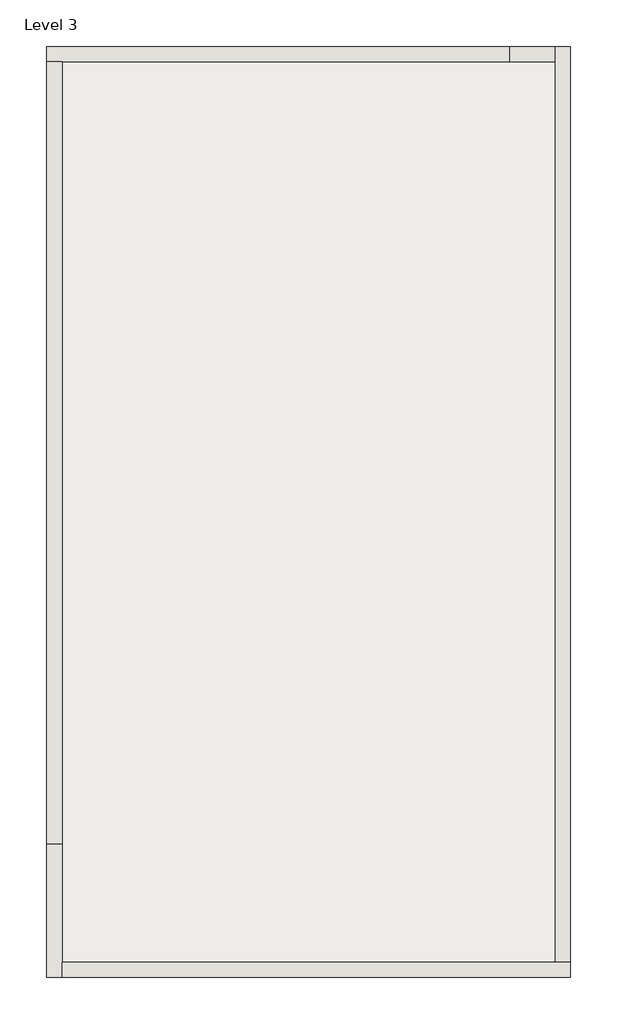
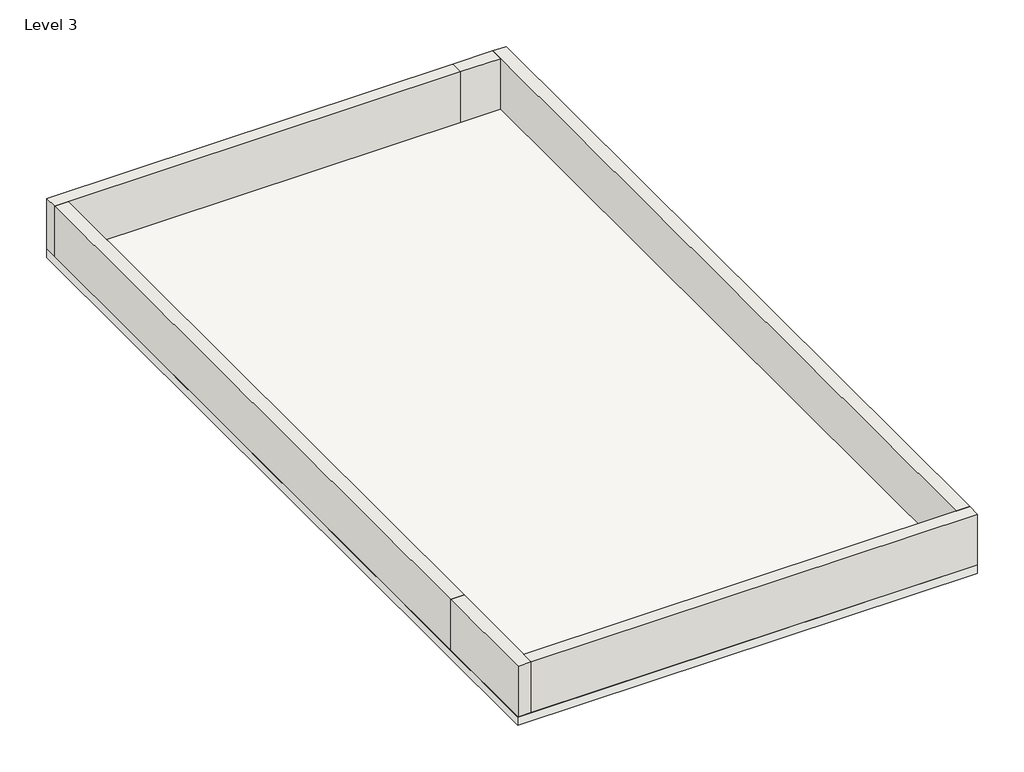
# One storey: 6 walls, 1 slab.
"""IFC4 building model written with IfcOpenShell, lengths in millimetres."""

from ifc_helpers import new_model, si_unit, frame, origin, place, context, project, spatial, polyline, outline, extrude, faceted_brep, element, save

model = new_model("IFC4")

# Units and contexts
model_context = context("Model", 3, world=origin())
ifc_project = project(units=[si_unit("LENGTHUNIT", "METRE", prefix="MILLI")], contexts=[model_context])

# Site, building, storey
site = spatial("IfcSite", under=ifc_project)
building = spatial("IfcBuilding", under=site)
storey = spatial("IfcBuildingStorey", under=building, Name="Level 3", Elevation=6400.8)

# Slab
placement = place(None, origin())
element("IfcSlab", 1, ObjectType="6\"", at=placement, inside=storey, context=model_context, shape_type="SweptSolid", body=[
    extrude(outline(polyline([(-1690.9371236, 5640.2122215), (-1690.9371236, -8304.3877785), (-9544.743556, -8304.3877785), (-9544.743556, 5640.2122215), (-1690.9371236, 5640.2122215)])), frame((0.0, 0.0, 6248.4), z_axis=(0.0, 0.0, 1.0), x_axis=(1.0, 0.0, 0.0)), (0.0, 0.0, 1.0), 152.4),
])

# Walls
element("IfcWall", 2, ObjectType="9\"", at=placement, inside=storey, context=model_context, shape_type="Brep", body=[
    faceted_brep([(-9538.393556, 5411.6122215, 6400.8), (-9309.793556, 5411.6122215, 6400.8), (-2604.193556, 5411.6122215, 6400.8), (-2604.193556, 5411.6122215, 7315.2), (-9309.793556, 5411.6122215, 7315.2), (-9538.393556, 5411.6122215, 7315.2), (-9538.393556, 5640.2122215, 6400.8), (-9538.393556, 5640.2122215, 7315.2), (-2604.193556, 5640.2122215, 7315.2), (-2604.193556, 5640.2122215, 6400.8)], [[[0, 1, 2, 3, 4, 5]], [[6, 7, 8, 9]], [[2, 1, 0, 6, 9]], [[3, 2, 9, 8]], [[5, 4, 3, 8, 7]], [[0, 5, 7, 6]]]),
])
element("IfcWall", 3, ObjectType="9\"", at=placement, inside=storey, context=model_context, shape_type="Brep", body=[
    faceted_brep([(-9309.793556, -8304.3877785, 6400.8), (-9309.793556, -8075.7877785, 6400.8), (-9309.793556, -6310.4877785, 6400.8), (-9309.793556, -6310.4877785, 7315.2), (-9309.793556, -8075.7877785, 7315.2), (-9309.793556, -8304.3877785, 7315.2), (-9538.393556, -8304.3877785, 6400.8), (-9538.393556, -8304.3877785, 7315.2), (-9538.393556, -6310.4877785, 7315.2), (-9538.393556, -6310.4877785, 6400.8)], [[[0, 1, 2, 3, 4, 5]], [[6, 7, 8, 9]], [[2, 1, 0, 6, 9]], [[3, 2, 9, 8]], [[5, 4, 3, 8, 7]], [[0, 5, 7, 6]]]),
])
element("IfcWall", 4, ObjectType="9\"", at=placement, inside=storey, context=model_context, shape_type="Brep", body=[
    faceted_brep([(-1689.793556, -8075.7877785, 6400.8), (-1918.393556, -8075.7877785, 6400.8), (-9309.793556, -8075.7877785, 6400.8), (-9309.793556, -8075.7877785, 7315.2), (-1918.393556, -8075.7877785, 7315.2), (-1689.793556, -8075.7877785, 7315.2), (-1689.793556, -8304.3877785, 6400.8), (-1689.793556, -8304.3877785, 7315.2), (-9309.793556, -8304.3877785, 7315.2), (-9309.793556, -8304.3877785, 6400.8)], [[[0, 1, 2, 3, 4, 5]], [[6, 7, 8, 9]], [[2, 1, 0, 6, 9]], [[5, 4, 3, 8, 7]], [[3, 2, 9, 8]], [[0, 5, 7, 6]]]),
])
element("IfcWall", 5, ObjectType="9\"", at=placement, inside=storey, context=model_context, shape_type="Brep", body=[
    faceted_brep([(-1918.393556, 5640.2122215, 6400.8), (-1918.393556, 5411.6122215, 6400.8), (-1918.393556, -8075.7877785, 6400.8), (-1918.393556, -8075.7877785, 7315.2), (-1918.393556, 5411.6122215, 7315.2), (-1918.393556, 5640.2122215, 7315.2), (-1689.793556, 5640.2122215, 6400.8), (-1689.793556, 5640.2122215, 7315.2), (-1689.793556, -8075.7877785, 7315.2), (-1689.793556, -8075.7877785, 6400.8)], [[[0, 1, 2, 3, 4, 5]], [[6, 7, 8, 9]], [[2, 1, 0, 6, 9]], [[5, 4, 3, 8, 7]], [[0, 5, 7, 6]], [[3, 2, 9, 8]]]),
])
element("IfcWall", 6, ObjectType="9\"", at=placement, inside=storey, context=model_context, shape_type="SweptSolid", body=[
    extrude(outline(polyline([(-9309.793556, 5411.6122215), (-9309.793556, -6310.4877785), (-9538.393556, -6310.4877785), (-9538.393556, 5411.6122215), (-9309.793556, 5411.6122215)])), frame((0.0, 0.0, 6400.8), z_axis=(0.0, 0.0, 1.0), x_axis=(1.0, 0.0, 0.0)), (0.0, 0.0, 1.0), 914.4),
])
element("IfcWall", 7, ObjectType="9\"", at=placement, inside=storey, context=model_context, shape_type="SweptSolid", body=[
    extrude(outline(polyline([(-1918.393556, 5411.6122215), (-2604.193556, 5411.6122215), (-2604.193556, 5640.2122215), (-1918.393556, 5640.2122215), (-1918.393556, 5411.6122215)])), frame((0.0, 0.0, 6400.8), z_axis=(0.0, 0.0, 1.0), x_axis=(1.0, 0.0, 0.0)), (0.0, 0.0, 1.0), 914.4),
])

save(model, "model.ifc")

# Revit data of these elements
# Type "6\""
#   Assembly Code = "B1010"
#   Function = 0
#   Layers, outside or top first: 0' - 6" "FLOOR" (function 1)
# Type "9\""
#   Assembly Code = "B2010"
#   Layers, outside or top first: 0' - 9" "EXT WALL" (function 1)
# Element 1 (IfcSlab, "6\"")
#   Height Offset From Level = 0' - 0"
#   Phase Created = New Construction
#   Materials on its faces: "FLOOR"
# Elements 2, 3, 4, 5, 6, 7 (IfcWall, "9\"")
#   Top Offset = 0' - 0"
#   Base Offset = 0' - 0"
#   Unconnected Height = 3' - 0"
#   wall height = 3' - 0"
#   Phase Created = New Construction
#   Base Constraint = Level 3
#   Materials on its faces: "EXT WALL"
# Materials
#   "FLOOR": class "Generic", colour RGB 144 129 110, transparency 0, Cost = 0
#   "EXT WALL": class "Generic", colour RGB 120 120 120, transparency 0, Cost = 0
